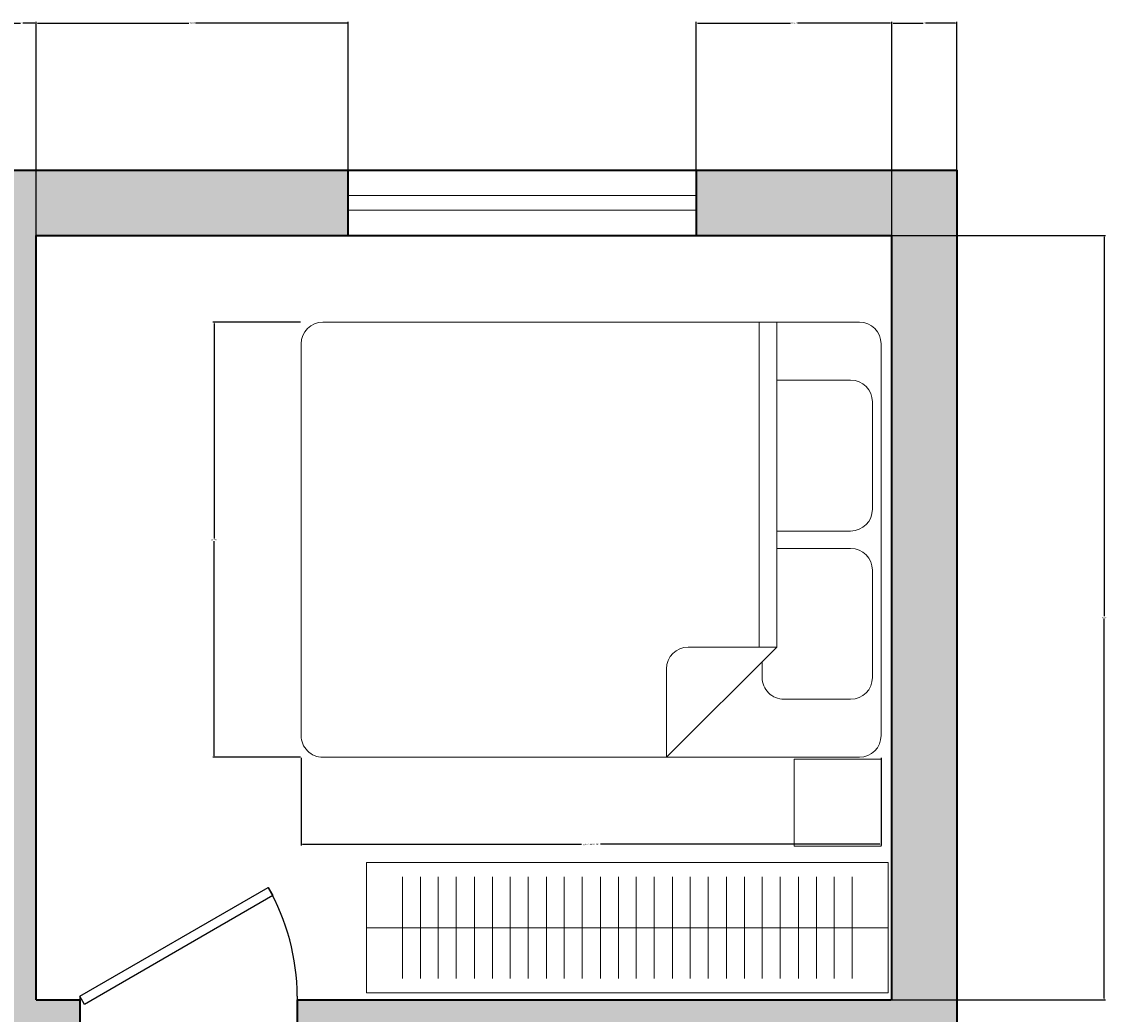
# Model space of a CAD drawing. Units: inches. Extents: x 1984 to 2284, y 2002 to 2421.
# Tile 4 of 4: x 2134 to 2283, y 2285 to 2421. Entities that reach past the tile are written whole.
import ezdxf

# ---------------------------------------------------------------- set-up
doc = ezdxf.new("R2010")
doc.units = ezdxf.units.IN
for name, color, linetype, lineweight in [('A-ANNO-DIMS', 2, 'Continuous', 18), ('A-DOOR', 3, 'Continuous', 25), ('A-FLOR-CASE', 9, 'Continuous', 20), ('A-FURN', 8, 'Continuous', 18), ('A-GLAZ', 4, 'Continuous', 18), ('A-WALL', 7, 'Continuous', 35)]:
    doc.layers.add(name, color=color, linetype=linetype, lineweight=lineweight)
doc.layers.add('A-WALL-PATT', color=18, linetype='Continuous', lineweight=13, true_color=0x000000)
doc.styles.get("Standard").update_dxf_attribs({"font": 'arial.ttf'})
doc.dimstyles.get("Standard").update_dxf_attribs({"dimtxt": 0.18, "dimasz": 0.18, "dimexe": 0.18, "dimexo": 0.0625, "dimgap": 0.09, "dimtad": 0, "dimtih": 1, "dimtoh": 1, "dimdec": 4, "dimzin": 0, "dimdsep": 46, "dimtxsty": 'Standard', "dimcen": 0.09, "dimadec": 0, "dimazin": 0, "dimtfac": 1, "dimtdec": 4, "dimtofl": 0, "dimtmove": 0, "dimatfit": 3, "dimfxl": 1, "dimtolj": 1, "dimtzin": 0, "dimarcsym": 0})

# ---------------------------------------------------------------- blocks, each defined once
blk = doc.blocks.new('Bed - Queen')
for p, q in [((3, 0), (56.99999, 0)), ((10.99999, -1.2), (25.79998, -1.2)), ((34.19999, -1.2), (48.99999, -1.2)), ((0, -77.00003), (0, -3)), ((7.99999, -14.4), (7.99999, -4.2)), ((28.79998, -4.2), (28.79998, -14.4)), ((31.19999, -14.4), (31.19999, -4.2)), ((51.99999, -4.2), (51.99999, -13.4)), ((59.99999, -3), (59.99999, -77.00003)), ((0, -14.4), (44.8, -14.4)), ((59.99999, -29.6), (44.8, -14.4)), ((44.8, -14.4), (44.8, -26.6)), ((48.99999, -16.4), (46.79936, -16.4)), ((44.8, -16.8), (0, -16.8)), ((47.8, -29.6), (59.99999, -29.6)), ((56.99999, -80.00003), (3, -80.00003))]:
    blk.add_line(p, q)
for centre, start, end in [((3, -3), 90, 180), ((56.99999, -3), 0, 90), ((10.99999, -4.2), 90, 180), ((25.79998, -4.2), 0, 90), ((34.19999, -4.2), 90, 180), ((48.99999, -4.2), 0, 90), ((48.99999, -13.4), 270, 0), ((47.8, -26.6), 180, 270), ((3, -77.00003), 180, 270), ((56.99999, -77.00003), 270, 0)]:
    blk.add_arc(centre, 3, start, end)
blk = doc.blocks.new('*U10')
for p, q in [((0, 0), (0, -6)), ((40, 0), (40, -6))]:
    blk.add_line(p, q)
blk.add_lwpolyline([(0, 0), (34.64, 20), (35.52, 18.48), (0.87, -1.52)], close=True)
blk.add_arc((0, 0), 40, 0, 30)
blk = doc.blocks.new('GLAZING-48IN')
for p, q in [((0, 2), (48, 2)), ((0, 0), (48, 0))]:
    blk.add_line(p, q)
blk = doc.blocks.new('WARDROBE-72IN')
for p, q in [((72, 18), (0, 18)), ((0, 18), (0, 0)), ((4.97, 16), (4.97, 2)), ((7.45, 16), (7.45, 2)), ((9.93, 16), (9.93, 2)), ((12.41, 16), (12.41, 2)), ((14.9, 16), (14.9, 2)), ((17.38, 16), (17.38, 2)), ((19.86, 16), (19.86, 2)), ((22.34, 16), (22.34, 2)), ((24.83, 16), (24.83, 2)), ((27.31, 16), (27.31, 2)), ((29.79, 16), (29.79, 2)), ((32.28, 16), (32.28, 2)), ((34.76, 16), (34.76, 2)), ((37.24, 16), (37.24, 2)), ((39.72, 16), (39.72, 2)), ((42.21, 16), (42.21, 2)), ((44.69, 16), (44.69, 2)), ((47.17, 16), (47.17, 2)), ((49.66, 16), (49.66, 2)), ((52.14, 16), (52.14, 2)), ((54.62, 16), (54.62, 2)), ((57.1, 16), (57.1, 2)), ((59.59, 16), (59.59, 2)), ((62.07, 16), (62.07, 2)), ((64.55, 16), (64.55, 2)), ((67.03, 16), (67.03, 2)), ((0, 9), (72, 9)), ((0, 0), (72, 0))]:
    blk.add_line(p, q)
blk.add_lwpolyline([(72, 18), (72, 0)], close=True)
blk = doc.blocks.new('NIGHTSTAND-12IN')
blk.add_lwpolyline([(0, 12), (12, 12), (12, 0), (0, 0)], close=True)
blk = doc.blocks.new('*D21')
at = {"layer": 'A-ANNO-DIMS', "color": 0, "lineweight": -2, "transparency": 16777216}
for p, q in [((2172.43, 2319.9), (2172.43, 2307.78)), ((2252.43, 2319.9), (2252.43, 2307.78)), ((2172.61, 2307.96), (2211.12, 2307.96)), ((2252.25, 2307.96), (2213.73, 2307.96))]:
    blk.add_line(p, q, dxfattribs=at)
at = {"layer": 'A-ANNO-DIMS', "color": 0, "transparency": 16777216}
for points in [[(2172.61, 2307.99), (2172.61, 2307.93), (2172.43, 2307.96)], [(2252.25, 2307.99), (2252.25, 2307.93), (2252.43, 2307.96)]]:
    blk.add_solid(points, dxfattribs=at)
at = {"layer": 'Defpoints', "color": 0, "transparency": 16777216}
for p in [(2172.43, 2319.96), (2252.43, 2319.96), (2252.43, 2307.96)]:
    blk.add_point(p, dxfattribs=at)
at = {"layer": 'A-ANNO-DIMS', "color": 0, "transparency": 16777216, "insert": (2212.43, 2307.96), "char_height": 0.18, "attachment_point": 5}
blk.add_mtext('\\A1;QUEEN BED 80 TYP.', dxfattribs=at)
blk = doc.blocks.new('*D22')
at = {"layer": 'A-ANNO-DIMS', "color": 0, "lineweight": -2, "transparency": 16777216}
for p, q in [((2172.36, 2379.96), (2160.25, 2379.96)), ((2160.43, 2379.78), (2160.43, 2350.14)), ((2160.43, 2320.14), (2160.43, 2349.78)), ((2172.36, 2319.96), (2160.25, 2319.96))]:
    blk.add_line(p, q, dxfattribs=at)
at = {"layer": 'A-ANNO-DIMS', "color": 0, "transparency": 16777216}
for points in [[(2160.4, 2379.78), (2160.46, 2379.78), (2160.43, 2379.96)], [(2160.4, 2320.14), (2160.46, 2320.14), (2160.43, 2319.96)]]:
    blk.add_solid(points, dxfattribs=at)
at = {"layer": 'Defpoints', "color": 0, "transparency": 16777216}
for p in [(2172.43, 2379.96), (2160.43, 2319.96), (2172.43, 2319.96)]:
    blk.add_point(p, dxfattribs=at)
at = {"layer": 'A-ANNO-DIMS', "color": 0, "transparency": 16777216, "insert": (2160.43, 2349.96), "char_height": 0.18, "attachment_point": 5}
blk.add_mtext('\\A1;60 TYP.', dxfattribs=at)
blk = doc.blocks.new('*D45')
at = {"layer": 'A-ANNO-DIMS', "color": 0, "lineweight": -2, "transparency": 16777216}
for p, q in [((2131.89, 2391.97), (2131.89, 2421.39)), ((2132.07, 2421.21), (2133.73, 2421.21)), ((2135.71, 2421.21), (2134.04, 2421.21)), ((2135.89, 2391.97), (2135.89, 2421.39))]:
    blk.add_line(p, q, dxfattribs=at)
at = {"layer": 'A-ANNO-DIMS', "color": 0, "transparency": 16777216}
for points in [[(2132.07, 2421.24), (2132.07, 2421.18), (2131.89, 2421.21)], [(2135.71, 2421.24), (2135.71, 2421.18), (2135.89, 2421.21)]]:
    blk.add_solid(points, dxfattribs=at)
at = {"layer": 'Defpoints', "color": 0, "transparency": 16777216}
for p in [(2135.89, 2421.21), (2131.89, 2391.91), (2135.89, 2391.91)]:
    blk.add_point(p, dxfattribs=at)
at = {"layer": 'A-ANNO-DIMS', "color": 0, "transparency": 16777216, "insert": (2133.89, 2421.21), "char_height": 0.18, "attachment_point": 5}
blk.add_mtext('\\A1;4', dxfattribs=at)
blk = doc.blocks.new('*D46')
at = {"layer": 'A-ANNO-DIMS', "color": 0, "lineweight": -2, "transparency": 16777216}
for p, q in [((2135.89, 2391.97), (2135.89, 2421.39)), ((2136.07, 2421.21), (2156.94, 2421.21)), ((2178.76, 2421.21), (2157.88, 2421.21)), ((2178.94, 2391.97), (2178.94, 2421.39))]:
    blk.add_line(p, q, dxfattribs=at)
at = {"layer": 'A-ANNO-DIMS', "color": 0, "transparency": 16777216}
for points in [[(2136.07, 2421.24), (2136.07, 2421.18), (2135.89, 2421.21)], [(2178.76, 2421.24), (2178.76, 2421.18), (2178.94, 2421.21)]]:
    blk.add_solid(points, dxfattribs=at)
at = {"layer": 'Defpoints', "color": 0, "transparency": 16777216}
for p in [(2178.94, 2421.21), (2135.89, 2391.91), (2178.94, 2391.91)]:
    blk.add_point(p, dxfattribs=at)
at = {"layer": 'A-ANNO-DIMS', "color": 0, "transparency": 16777216, "insert": (2157.41, 2421.21), "char_height": 0.18, "attachment_point": 5}
blk.add_mtext('\\A1;43.055', dxfattribs=at)
blk = doc.blocks.new('*D47')
at = {"layer": 'A-ANNO-DIMS', "color": 0, "lineweight": -2, "transparency": 16777216}
for p, q in [((2226.94, 2391.97), (2226.94, 2421.39)), ((2227.12, 2421.21), (2239.95, 2421.21)), ((2253.71, 2421.21), (2240.88, 2421.21)), ((2253.89, 2391.97), (2253.89, 2421.39))]:
    blk.add_line(p, q, dxfattribs=at)
at = {"layer": 'A-ANNO-DIMS', "color": 0, "transparency": 16777216}
for points in [[(2227.12, 2421.24), (2227.12, 2421.18), (2226.94, 2421.21)], [(2253.71, 2421.24), (2253.71, 2421.18), (2253.89, 2421.21)]]:
    blk.add_solid(points, dxfattribs=at)
at = {"layer": 'Defpoints', "color": 0, "transparency": 16777216}
for p in [(2253.89, 2421.21), (2226.94, 2391.91), (2253.89, 2391.91)]:
    blk.add_point(p, dxfattribs=at)
at = {"layer": 'A-ANNO-DIMS', "color": 0, "transparency": 16777216, "insert": (2240.41, 2421.21), "char_height": 0.18, "attachment_point": 5}
blk.add_mtext('\\A1;26.945', dxfattribs=at)
blk = doc.blocks.new('*D48')
at = {"layer": 'A-ANNO-DIMS', "color": 0, "lineweight": -2, "transparency": 16777216}
for p, q in [((2253.89, 2391.97), (2253.89, 2421.39)), ((2254.07, 2421.21), (2258.24, 2421.21)), ((2262.71, 2421.21), (2258.53, 2421.21)), ((2262.89, 2400.97), (2262.89, 2421.39))]:
    blk.add_line(p, q, dxfattribs=at)
at = {"layer": 'A-ANNO-DIMS', "color": 0, "transparency": 16777216}
for points in [[(2254.07, 2421.24), (2254.07, 2421.18), (2253.89, 2421.21)], [(2262.71, 2421.24), (2262.71, 2421.18), (2262.89, 2421.21)]]:
    blk.add_solid(points, dxfattribs=at)
at = {"layer": 'Defpoints', "color": 0, "transparency": 16777216}
for p in [(2262.89, 2421.21), (2262.89, 2400.91), (2253.89, 2391.91)]:
    blk.add_point(p, dxfattribs=at)
at = {"layer": 'A-ANNO-DIMS', "color": 0, "transparency": 16777216, "insert": (2258.39, 2421.21), "char_height": 0.18, "attachment_point": 5}
blk.add_mtext('\\A1;9', dxfattribs=at)
blk = doc.blocks.new('*D50')
at = {"layer": 'A-ANNO-DIMS', "color": 0, "lineweight": -2, "transparency": 16777216}
for p, q in [((2253.95, 2391.91), (2283.37, 2391.91)), ((2283.19, 2391.73), (2283.19, 2339.4)), ((2283.19, 2286.69), (2283.19, 2339.03)), ((2253.95, 2286.51), (2283.37, 2286.51))]:
    blk.add_line(p, q, dxfattribs=at)
at = {"layer": 'A-ANNO-DIMS', "color": 0, "transparency": 16777216}
for points in [[(2283.16, 2391.73), (2283.22, 2391.73), (2283.19, 2391.91)], [(2283.16, 2286.69), (2283.22, 2286.69), (2283.19, 2286.51)]]:
    blk.add_solid(points, dxfattribs=at)
at = {"layer": 'Defpoints', "color": 0, "transparency": 16777216}
for p in [(2253.89, 2391.91), (2253.89, 2286.51), (2283.19, 2286.51)]:
    blk.add_point(p, dxfattribs=at)
at = {"layer": 'A-ANNO-DIMS', "color": 0, "transparency": 16777216, "insert": (2283.19, 2339.21), "char_height": 0.18, "attachment_point": 5}
blk.add_mtext('\\A1;105.4', dxfattribs=at)

msp = doc.modelspace()

# ---------------------------------------------------------------- hatches: boundary and pattern name
at = {"layer": 'A-WALL-PATT'}
h = msp.add_hatch(color=256, dxfattribs=at)
h.dxf.hatch_style = 1
h.paths.add_polyline_path([(2178.9401, 2400.9122), (2100.8198, 2400.9122), (2100.8198, 2391.9122), (2131.8852, 2391.9122), (2131.8852, 2271.9122), (2125.8852, 2271.9122), (2125.8852, 2267.9122), (2135.8852, 2267.9122), (2135.8852, 2271.9122), (2135.8852, 2282.5141), (2141.8852, 2282.5141), (2141.8852, 2286.5141), (2135.8852, 2286.5141), (2135.8852, 2391.9122), (2178.9401, 2391.9122)])
h = msp.add_hatch(color=256, dxfattribs=at)
h.dxf.hatch_style = 1
h.paths.add_polyline_path([(2262.8852, 2400.9122), (2226.9401, 2400.9122), (2226.9401, 2391.9122), (2253.8852, 2391.9122), (2253.8852, 2286.5141), (2171.8852, 2286.5141), (2171.8852, 2282.5141), (2177.8852, 2282.5141), (2177.8852, 2276.5141), (2181.8852, 2276.5141), (2181.8852, 2282.5141), (2253.8852, 2282.5141), (2253.8852, 2255.5995), (2262.8852, 2255.5995)])

# ---------------------------------------------------------------- linework, layer by layer
at = {"layer": 'A-WALL'}
for p, q in [((2135.8852, 2391.9122), (2253.8852, 2391.9122)), ((2135.8852, 2286.5141), (2135.8852, 2391.9122)), ((2253.8852, 2391.9122), (2253.8852, 2286.5141)), ((2135.8852, 2286.5141), (2141.8852, 2286.5141)), ((2141.8852, 2286.5141), (2141.8852, 2282.5141)), ((2171.8852, 2286.5141), (2171.8852, 2282.5141)), ((2171.8852, 2286.5141), (2253.8852, 2286.5141))]:
    msp.add_line(p, q, dxfattribs=at)
for points in [[(2019.8852, 2022.9122), (2004.8852, 2022.9122), (2004.8852, 2400.9122), (2262.8852, 2400.9122), (2262.8852, 2022.9122), (2055.8852, 2022.9122)], [(2178.9401, 2391.9122), (2178.9401, 2400.9122)], [(2226.9401, 2400.9122), (2226.9401, 2391.9122)]]:
    msp.add_lwpolyline(points, dxfattribs=at)

# ---------------------------------------------------------------- block references
at = {"layer": 'A-DOOR', "xscale": 0.75, "yscale": 0.75, "zscale": 0.75}
msp.add_blockref('*U10', (2141.8852, 2287.0141), dxfattribs=at)
at = {"layer": 'A-FLOR-CASE'}
msp.add_blockref('WARDROBE-72IN', (2181.4243, 2287.4602), dxfattribs=at)
at = {"layer": 'A-FURN', "rotation": 270}
msp.add_blockref('Bed - Queen', (2252.4255, 2379.9577), dxfattribs=at)
at = {"layer": 'A-FURN'}
msp.add_blockref('NIGHTSTAND-12IN', (2240.4145, 2307.6777), dxfattribs=at)
at = {"layer": 'A-GLAZ'}
msp.add_blockref('GLAZING-48IN', (2178.9401, 2395.4122), dxfattribs=at)

# ---------------------------------------------------------------- dimensions: what is measured, and where the dimension line sits
at = {"layer": 'A-ANNO-DIMS'}
for base, p1, p2, override, picture, middle in [((2135.8852, 2421.2122), (2131.8852, 2391.9122), (2135.8852, 2391.9122), {"dimdec": 0, "dimlfac": 1, "dimrnd": 0, "dimzin": 0, "dimdsep": 46, "dimlunit": 2}, '*D45', (2133.8852, 2421.2122)), ((2178.9401, 2421.2122), (2135.8852, 2391.9122), (2178.9401, 2391.9122), {"dimdec": 3, "dimlfac": 1, "dimrnd": 0, "dimzin": 0, "dimdsep": 46, "dimlunit": 2}, '*D46', (2157.4127, 2421.2122)), ((2253.8852, 2421.2122), (2226.9401, 2391.9122), (2253.8852, 2391.9122), {"dimdec": 3, "dimlfac": 1, "dimrnd": 0, "dimzin": 0, "dimdsep": 46, "dimlunit": 2}, '*D47', (2240.4127, 2421.2122)), ((2262.8852, 2421.2122), (2253.8852, 2391.9122), (2262.8852, 2400.9122), {"dimdec": 0, "dimlfac": 1, "dimrnd": 0, "dimzin": 0, "dimdsep": 46, "dimlunit": 2}, '*D48', (2258.3852, 2421.2122))]:
    dim = msp.add_linear_dim(base=base, p1=p1, p2=p2, dimstyle='Standard', override=override, dxfattribs=at)
    dim.commit()
    dim.dimension.update_dxf_attribs({"geometry": picture, "text_midpoint": middle})
dim = msp.add_linear_dim(base=(2283.1852, 2286.5141), p1=(2253.8852, 2391.9122), p2=(2253.8852, 2286.5141), angle=90, dimstyle='Standard', override={"dimdec": 1, "dimlfac": 1, "dimrnd": 0, "dimzin": 0, "dimdsep": 46, "dimlunit": 2}, dxfattribs=at)
dim.commit()
dim.dimension.update_dxf_attribs({"geometry": '*D50', "text_midpoint": (2283.1852, 2339.2132)})
dim = msp.add_linear_dim(base=(2160.4254, 2319.9577), p1=(2172.4254, 2379.9577), p2=(2172.4254, 2319.9577), angle=270, text='<> TYP.', dimstyle='Standard', override={"dimdec": 0, "dimlfac": 1, "dimrnd": 0, "dimzin": 0, "dimdsep": 46, "dimlunit": 2}, dxfattribs=at)
dim.commit()
dim.dimension.update_dxf_attribs({"geometry": '*D22', "text_midpoint": (2160.4254, 2349.9577)})
dim = msp.add_linear_dim(base=(2252.4255, 2307.9577), p1=(2172.4254, 2319.9577), p2=(2252.4255, 2319.9577), text='QUEEN BED <> TYP.', dimstyle='Standard', override={"dimdec": 0, "dimlfac": 1, "dimrnd": 0, "dimzin": 0, "dimdsep": 46, "dimlunit": 2}, dxfattribs=at)
dim.commit()
dim.dimension.update_dxf_attribs({"geometry": '*D21', "text_midpoint": (2212.4254, 2307.9577)})

doc.saveas('drawing.dxf')
